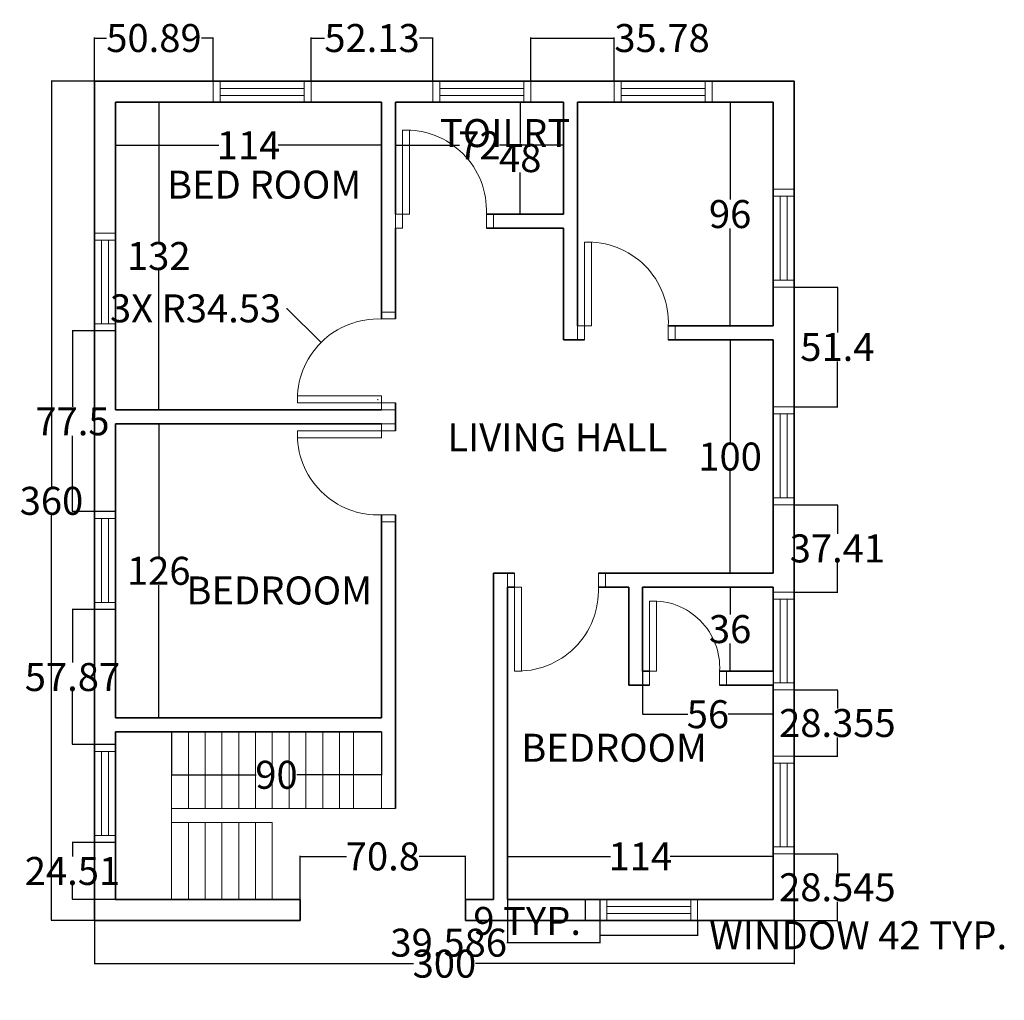
# Model space of a CAD drawing. Units: inches. Extents: x -24 to 1692, y -109 to 592.
# Tile 4 of 4: x 1270 to 1692, y 17 to 437. Entities that reach past the tile are written whole.
import ezdxf
from ezdxf.enums import TextEntityAlignment as Align

# ---------------------------------------------------------------- set-up
doc = ezdxf.new("R2010")
doc.units = ezdxf.units.IN
doc.header["$MEASUREMENT"] = 0
for name, color, linetype, lineweight in [('A-ANNO-DIMS', 2, 'Continuous', 18), ('A-AREA-IDEN', 7, 'Continuous', 18), ('A-DOOR', 3, 'Continuous', 18), ('A-FLOR-STRS', 2, 'Continuous', 18), ('A-GLAZ', 4, 'Continuous', 18), ('A-WALL', 7, 'Continuous', 35)]:
    doc.layers.add(name, color=color, linetype=linetype, lineweight=lineweight)
doc.styles.get("Standard").update_dxf_attribs({"font": 'arial.ttf'})
doc.dimstyles.get("Standard").update_dxf_attribs({"dimtxt": 12, "dimasz": 0.18, "dimexe": 0.18, "dimexo": 0.0625, "dimgap": 0.09, "dimtad": 0, "dimtih": 1, "dimtoh": 1, "dimdec": 0, "dimzin": 0, "dimdsep": 46, "dimlunit": 4, "dimtxsty": 'Standard', "dimcen": 0.09, "dimadec": 0, "dimazin": 0, "dimtfac": 1, "dimtdec": 0, "dimtofl": 0, "dimtmove": 0, "dimatfit": 3, "dimfxl": 1, "dimtolj": 1, "dimtzin": 0, "dimarcsym": 0})

# ---------------------------------------------------------------- blocks, each defined once
blk = doc.blocks.new('K')
for p, q in [((0, 42), (9, 42)), ((0, 3), (0, 39)), ((0, 39), (9, 39)), ((3, 3), (3, 39)), ((6, 39), (6, 3)), ((9, 39), (9, 3)), ((9, 3), (0, 3)), ((9, 0), (0, 0))]:
    blk.add_line(p, q)
blk = doc.blocks.new('DOOR-SWING-36IN')
for p, q in [((-39, 0), (-39, 6)), ((-36, 0), (-36, 6)), ((0, 0), (0, 6)), ((3, 0), (3, 6))]:
    blk.add_line(p, q)
blk.add_lwpolyline([(0, 0), (-3, 0), (-3, -36), (0, -36)], close=True)
blk.add_arc((-1.5, -1.5), 34.53, 177.5104, 272.4896)
blk = doc.blocks.new('DOOR-SWING-30IN')
for p, q in [((-3, 6), (-3, 0)), ((0, 6), (0, 0)), ((30, 6), (30, 0)), ((33, 6), (33, 0))]:
    blk.add_line(p, q)
blk.add_lwpolyline([(0, 0), (3, 0), (3, -30), (0, -30)], close=True)
blk.add_arc((1.5, -1.5), 28.54, 266.9872, 3.0128)
blk = doc.blocks.new('*D5')
at = {"layer": 'A-ANNO-DIMS', "color": 0, "lineweight": -2, "transparency": 16777216}
for p, q in [((1519, 51.05), (1519, 44.64)), ((1561, 51.05), (1561, 44.64)), ((1519.18, 44.82), (1560.82, 44.82)), ((1561, 44.82), (1561.18, 44.82))]:
    blk.add_line(p, q, dxfattribs=at)
at = {"layer": 'A-ANNO-DIMS', "color": 0, "transparency": 16777216}
for points in [[(1519.18, 44.85), (1519.18, 44.79), (1519, 44.82)], [(1560.82, 44.85), (1560.82, 44.79), (1561, 44.82)]]:
    blk.add_solid(points, dxfattribs=at)
at = {"layer": 'Defpoints', "color": 0, "transparency": 16777216}
for p in [(1519, 51.12), (1561, 51.12), (1561, 44.82)]:
    blk.add_point(p, dxfattribs=at)
at = {"layer": 'A-ANNO-DIMS', "color": 0, "transparency": 16777216, "insert": (1629.83, 44.82), "char_height": 12, "attachment_point": 5}
blk.add_mtext('\\A1;WINDOW 42 TYP.', dxfattribs=at)
blk = doc.blocks.new('*D6')
at = {"layer": 'A-ANNO-DIMS', "color": 0, "lineweight": -2, "transparency": 16777216}
for p, q in [((1518.94, 60.12), (1512.52, 60.12)), ((1512.7, 59.94), (1512.7, 51.3)), ((1518.94, 51.12), (1512.52, 51.12)), ((1512.7, 50.94), (1512.52, 50.94)), ((1512.7, 51.12), (1512.7, 50.94))]:
    blk.add_line(p, q, dxfattribs=at)
at = {"layer": 'A-ANNO-DIMS', "color": 0, "transparency": 16777216}
for points in [[(1512.67, 59.94), (1512.73, 59.94), (1512.7, 60.12)], [(1512.67, 51.3), (1512.73, 51.3), (1512.7, 51.12)]]:
    blk.add_solid(points, dxfattribs=at)
at = {"layer": 'Defpoints', "color": 0, "transparency": 16777216}
for p in [(1519, 60.12), (1512.7, 51.12), (1519, 51.12)]:
    blk.add_point(p, dxfattribs=at)
at = {"layer": 'A-ANNO-DIMS', "color": 0, "transparency": 16777216, "insert": (1487.89, 50.94), "char_height": 12, "attachment_point": 5}
blk.add_mtext('\\A1;9 TYP.', dxfattribs=at)
blk = doc.blocks.new('*D72')
at = {"layer": 'A-ANNO-DIMS', "color": 0, "lineweight": -2, "transparency": 16777216}
for p, q in [((1302.41, 51.05), (1302.41, 32.44)), ((1602.41, 51.05), (1602.41, 32.44)), ((1302.59, 32.62), (1439.09, 32.62)), ((1602.23, 32.62), (1465.74, 32.62))]:
    blk.add_line(p, q, dxfattribs=at)
at = {"layer": 'A-ANNO-DIMS', "color": 0, "transparency": 16777216}
for points in [[(1302.59, 32.65), (1302.59, 32.59), (1302.41, 32.62)], [(1602.23, 32.65), (1602.23, 32.59), (1602.41, 32.62)]]:
    blk.add_solid(points, dxfattribs=at)
at = {"layer": 'Defpoints', "color": 0, "transparency": 16777216}
for p in [(1302.41, 51.12), (1602.41, 51.12), (1602.41, 32.62)]:
    blk.add_point(p, dxfattribs=at)
at = {"layer": 'A-ANNO-DIMS', "color": 0, "transparency": 16777216, "insert": (1452.41, 32.62), "char_height": 12, "attachment_point": 5}
blk.add_mtext('\\A1;300', dxfattribs=at)
blk = doc.blocks.new('*D73')
at = {"layer": 'A-ANNO-DIMS', "color": 0, "lineweight": -2, "transparency": 16777216}
for p, q in [((1302.35, 411.12), (1283.73, 411.12)), ((1283.91, 410.94), (1283.91, 237.34)), ((1283.91, 51.3), (1283.91, 224.89)), ((1302.35, 51.12), (1283.73, 51.12))]:
    blk.add_line(p, q, dxfattribs=at)
at = {"layer": 'A-ANNO-DIMS', "color": 0, "transparency": 16777216}
for points in [[(1283.88, 410.94), (1283.94, 410.94), (1283.91, 411.12)], [(1283.88, 51.3), (1283.94, 51.3), (1283.91, 51.12)]]:
    blk.add_solid(points, dxfattribs=at)
at = {"layer": 'Defpoints', "color": 0, "transparency": 16777216}
for p in [(1283.91, 411.12), (1302.41, 411.12), (1302.41, 51.12)]:
    blk.add_point(p, dxfattribs=at)
at = {"layer": 'A-ANNO-DIMS', "color": 0, "transparency": 16777216, "insert": (1283.91, 231.12), "char_height": 12, "attachment_point": 5}
blk.add_mtext('\\A1;360', dxfattribs=at)
blk = doc.blocks.new('*D74')
at = {"layer": 'A-ANNO-DIMS', "color": 0, "lineweight": -2, "transparency": 16777216}
for p, q in [((1311.41, 402.05), (1311.41, 383.44)), ((1425.41, 402.05), (1425.41, 383.44)), ((1311.59, 383.62), (1355.66, 383.62)), ((1425.23, 383.62), (1381.17, 383.62))]:
    blk.add_line(p, q, dxfattribs=at)
at = {"layer": 'A-ANNO-DIMS', "color": 0, "transparency": 16777216}
for points in [[(1311.59, 383.65), (1311.59, 383.59), (1311.41, 383.62)], [(1425.23, 383.65), (1425.23, 383.59), (1425.41, 383.62)]]:
    blk.add_solid(points, dxfattribs=at)
at = {"layer": 'Defpoints', "color": 0, "transparency": 16777216}
for p in [(1311.41, 402.12), (1425.41, 402.12), (1311.41, 383.62)]:
    blk.add_point(p, dxfattribs=at)
at = {"layer": 'A-ANNO-DIMS', "color": 0, "transparency": 16777216, "insert": (1368.41, 383.62), "char_height": 12, "attachment_point": 5}
blk.add_mtext('\\A1;114', dxfattribs=at)
blk = doc.blocks.new('*D75')
at = {"layer": 'A-ANNO-DIMS', "color": 0, "lineweight": -2, "transparency": 16777216}
for p, q in [((1431.41, 402.05), (1431.41, 383.44)), ((1503.41, 402.05), (1503.41, 383.44)), ((1431.59, 383.62), (1458.84, 383.62)), ((1503.23, 383.62), (1475.99, 383.62))]:
    blk.add_line(p, q, dxfattribs=at)
at = {"layer": 'A-ANNO-DIMS', "color": 0, "transparency": 16777216}
for points in [[(1431.59, 383.65), (1431.59, 383.59), (1431.41, 383.62)], [(1503.23, 383.65), (1503.23, 383.59), (1503.41, 383.62)]]:
    blk.add_solid(points, dxfattribs=at)
at = {"layer": 'Defpoints', "color": 0, "transparency": 16777216}
for p in [(1431.41, 402.12), (1503.41, 402.12), (1431.41, 383.62)]:
    blk.add_point(p, dxfattribs=at)
at = {"layer": 'A-ANNO-DIMS', "color": 0, "transparency": 16777216, "insert": (1467.41, 383.62), "char_height": 12, "attachment_point": 5}
blk.add_mtext('\\A1;72', dxfattribs=at)
blk = doc.blocks.new('*D76')
at = {"layer": 'A-ANNO-DIMS', "color": 0, "lineweight": -2, "transparency": 16777216}
for p, q in [((1311.48, 402.12), (1330.09, 402.12)), ((1329.91, 401.94), (1329.91, 342.34)), ((1329.91, 270.3), (1329.91, 329.89)), ((1311.48, 270.12), (1330.09, 270.12))]:
    blk.add_line(p, q, dxfattribs=at)
at = {"layer": 'A-ANNO-DIMS', "color": 0, "transparency": 16777216}
for points in [[(1329.88, 401.94), (1329.94, 401.94), (1329.91, 402.12)], [(1329.88, 270.3), (1329.94, 270.3), (1329.91, 270.12)]]:
    blk.add_solid(points, dxfattribs=at)
at = {"layer": 'Defpoints', "color": 0, "transparency": 16777216}
for p in [(1311.41, 402.12), (1311.41, 270.12), (1329.91, 270.12)]:
    blk.add_point(p, dxfattribs=at)
at = {"layer": 'A-ANNO-DIMS', "color": 0, "transparency": 16777216, "insert": (1329.91, 336.12), "char_height": 12, "attachment_point": 5}
blk.add_mtext('\\A1;132', dxfattribs=at)
blk = doc.blocks.new('*D77')
at = {"layer": 'A-ANNO-DIMS', "color": 0, "lineweight": -2, "transparency": 16777216}
for p, q in [((1311.48, 264.12), (1330.09, 264.12)), ((1329.91, 263.94), (1329.91, 207.33)), ((1329.91, 138.3), (1329.91, 194.9)), ((1311.48, 138.12), (1330.09, 138.12))]:
    blk.add_line(p, q, dxfattribs=at)
at = {"layer": 'A-ANNO-DIMS', "color": 0, "transparency": 16777216}
for points in [[(1329.88, 263.94), (1329.94, 263.94), (1329.91, 264.12)], [(1329.88, 138.3), (1329.94, 138.3), (1329.91, 138.12)]]:
    blk.add_solid(points, dxfattribs=at)
at = {"layer": 'Defpoints', "color": 0, "transparency": 16777216}
for p in [(1311.41, 264.12), (1311.41, 138.12), (1329.91, 138.12)]:
    blk.add_point(p, dxfattribs=at)
at = {"layer": 'A-ANNO-DIMS', "color": 0, "transparency": 16777216, "insert": (1329.91, 201.12), "char_height": 12, "attachment_point": 5}
blk.add_mtext('\\A1;126', dxfattribs=at)
blk = doc.blocks.new('*D78')
at = {"layer": 'A-ANNO-DIMS', "color": 0, "lineweight": -2, "transparency": 16777216}
for p, q in [((1593.35, 402.12), (1574.73, 402.12)), ((1574.91, 401.94), (1574.91, 360.33)), ((1574.91, 306.3), (1574.91, 347.9)), ((1593.35, 306.12), (1574.73, 306.12))]:
    blk.add_line(p, q, dxfattribs=at)
at = {"layer": 'A-ANNO-DIMS', "color": 0, "transparency": 16777216}
for points in [[(1574.88, 401.94), (1574.94, 401.94), (1574.91, 402.12)], [(1574.88, 306.3), (1574.94, 306.3), (1574.91, 306.12)]]:
    blk.add_solid(points, dxfattribs=at)
at = {"layer": 'Defpoints', "color": 0, "transparency": 16777216}
for p in [(1574.91, 402.12), (1593.41, 402.12), (1593.41, 306.12)]:
    blk.add_point(p, dxfattribs=at)
at = {"layer": 'A-ANNO-DIMS', "color": 0, "transparency": 16777216, "insert": (1574.91, 354.12), "char_height": 12, "attachment_point": 5}
blk.add_mtext('\\A1;96', dxfattribs=at)
blk = doc.blocks.new('*D79')
at = {"layer": 'A-ANNO-DIMS', "color": 0, "lineweight": -2, "transparency": 16777216}
for p, q in [((1593.35, 300.12), (1574.73, 300.12)), ((1574.91, 299.94), (1574.91, 256.33)), ((1574.91, 200.3), (1574.91, 243.9)), ((1593.35, 200.12), (1574.73, 200.12))]:
    blk.add_line(p, q, dxfattribs=at)
at = {"layer": 'A-ANNO-DIMS', "color": 0, "transparency": 16777216}
for points in [[(1574.88, 299.94), (1574.94, 299.94), (1574.91, 300.12)], [(1574.88, 200.3), (1574.94, 200.3), (1574.91, 200.12)]]:
    blk.add_solid(points, dxfattribs=at)
at = {"layer": 'Defpoints', "color": 0, "transparency": 16777216}
for p in [(1574.91, 300.12), (1593.41, 300.12), (1593.41, 200.12)]:
    blk.add_point(p, dxfattribs=at)
at = {"layer": 'A-ANNO-DIMS', "color": 0, "transparency": 16777216, "insert": (1574.91, 250.12), "char_height": 12, "attachment_point": 5}
blk.add_mtext('\\A1;100', dxfattribs=at)
blk = doc.blocks.new('*D80')
at = {"layer": 'A-ANNO-DIMS', "color": 0, "lineweight": -2, "transparency": 16777216}
for p, q in [((1503.35, 402.12), (1484.73, 402.12)), ((1484.91, 401.94), (1484.91, 384.33)), ((1484.91, 354.3), (1484.91, 371.9)), ((1503.35, 354.12), (1484.73, 354.12))]:
    blk.add_line(p, q, dxfattribs=at)
at = {"layer": 'A-ANNO-DIMS', "color": 0, "transparency": 16777216}
for points in [[(1484.88, 401.94), (1484.94, 401.94), (1484.91, 402.12)], [(1484.88, 354.3), (1484.94, 354.3), (1484.91, 354.12)]]:
    blk.add_solid(points, dxfattribs=at)
at = {"layer": 'Defpoints', "color": 0, "transparency": 16777216}
for p in [(1484.91, 402.12), (1503.41, 402.12), (1503.41, 354.12)]:
    blk.add_point(p, dxfattribs=at)
at = {"layer": 'A-ANNO-DIMS', "color": 0, "transparency": 16777216, "insert": (1484.91, 378.12), "char_height": 12, "attachment_point": 5}
blk.add_mtext('\\A1;48', dxfattribs=at)
blk = doc.blocks.new('*D81')
at = {"layer": 'A-ANNO-DIMS', "color": 0, "lineweight": -2, "transparency": 16777216}
for p, q in [((1479.41, 60.18), (1479.41, 78.8)), ((1479.59, 78.62), (1523.66, 78.62)), ((1593.23, 78.62), (1549.17, 78.62)), ((1593.41, 60.18), (1593.41, 78.8))]:
    blk.add_line(p, q, dxfattribs=at)
at = {"layer": 'A-ANNO-DIMS', "color": 0, "transparency": 16777216}
for points in [[(1479.59, 78.65), (1479.59, 78.59), (1479.41, 78.62)], [(1593.23, 78.65), (1593.23, 78.59), (1593.41, 78.62)]]:
    blk.add_solid(points, dxfattribs=at)
at = {"layer": 'Defpoints', "color": 0, "transparency": 16777216}
for p in [(1593.41, 78.62), (1479.41, 60.12), (1593.41, 60.12)]:
    blk.add_point(p, dxfattribs=at)
at = {"layer": 'A-ANNO-DIMS', "color": 0, "transparency": 16777216, "insert": (1536.41, 78.62), "char_height": 12, "attachment_point": 5}
blk.add_mtext('\\A1;114', dxfattribs=at)
blk = doc.blocks.new('*D82')
at = {"layer": 'A-ANNO-DIMS', "color": 0, "lineweight": -2, "transparency": 16777216}
for p, q in [((1390.61, 60.18), (1390.61, 78.8)), ((1390.79, 78.62), (1410.38, 78.62)), ((1461.23, 78.62), (1441.65, 78.62)), ((1461.41, 60.18), (1461.41, 78.8))]:
    blk.add_line(p, q, dxfattribs=at)
at = {"layer": 'A-ANNO-DIMS', "color": 0, "transparency": 16777216}
for points in [[(1390.79, 78.65), (1390.79, 78.59), (1390.61, 78.62)], [(1461.23, 78.65), (1461.23, 78.59), (1461.41, 78.62)]]:
    blk.add_solid(points, dxfattribs=at)
at = {"layer": 'Defpoints', "color": 0, "transparency": 16777216}
for p in [(1461.41, 78.62), (1390.61, 60.12), (1461.41, 60.12)]:
    blk.add_point(p, dxfattribs=at)
at = {"layer": 'A-ANNO-DIMS', "color": 0, "transparency": 16777216, "insert": (1426.01, 78.62), "char_height": 12, "attachment_point": 5}
blk.add_mtext('\\A1;70.8', dxfattribs=at)
blk = doc.blocks.new('*D83')
at = {"layer": 'A-ANNO-DIMS', "color": 0, "lineweight": -2, "transparency": 16777216}
for p, q in [((1537.41, 158.05), (1537.41, 139.44)), ((1593.41, 158.05), (1593.41, 139.44)), ((1537.59, 139.62), (1556.73, 139.62)), ((1593.23, 139.62), (1574.09, 139.62))]:
    blk.add_line(p, q, dxfattribs=at)
at = {"layer": 'A-ANNO-DIMS', "color": 0, "transparency": 16777216}
for points in [[(1537.59, 139.65), (1537.59, 139.59), (1537.41, 139.62)], [(1593.23, 139.65), (1593.23, 139.59), (1593.41, 139.62)]]:
    blk.add_solid(points, dxfattribs=at)
at = {"layer": 'Defpoints', "color": 0, "transparency": 16777216}
for p in [(1537.41, 158.12), (1593.41, 158.12), (1537.41, 139.62)]:
    blk.add_point(p, dxfattribs=at)
at = {"layer": 'A-ANNO-DIMS', "color": 0, "transparency": 16777216, "insert": (1565.41, 139.62), "char_height": 12, "attachment_point": 5}
blk.add_mtext('\\A1;56', dxfattribs=at)
blk = doc.blocks.new('*D84')
at = {"layer": 'A-ANNO-DIMS', "color": 0, "lineweight": -2, "transparency": 16777216}
for p, q in [((1593.35, 194.12), (1574.73, 194.12)), ((1574.91, 193.94), (1574.91, 182.34)), ((1574.91, 158.3), (1574.91, 169.89)), ((1593.35, 158.12), (1574.73, 158.12))]:
    blk.add_line(p, q, dxfattribs=at)
at = {"layer": 'A-ANNO-DIMS', "color": 0, "transparency": 16777216}
for points in [[(1574.88, 193.94), (1574.94, 193.94), (1574.91, 194.12)], [(1574.88, 158.3), (1574.94, 158.3), (1574.91, 158.12)]]:
    blk.add_solid(points, dxfattribs=at)
at = {"layer": 'Defpoints', "color": 0, "transparency": 16777216}
for p in [(1574.91, 194.12), (1593.41, 194.12), (1593.41, 158.12)]:
    blk.add_point(p, dxfattribs=at)
at = {"layer": 'A-ANNO-DIMS', "color": 0, "transparency": 16777216, "insert": (1574.91, 176.12), "char_height": 12, "attachment_point": 5}
blk.add_mtext('\\A1;36', dxfattribs=at)
blk = doc.blocks.new('*D85')
at = {"layer": 'A-ANNO-DIMS', "color": 0, "lineweight": -2, "transparency": 16777216}
for p, q in [((1302.41, 411.18), (1302.41, 429.8)), ((1302.59, 429.62), (1307.51, 429.62)), ((1353.12, 429.62), (1348.21, 429.62)), ((1353.3, 411.07), (1353.3, 429.8))]:
    blk.add_line(p, q, dxfattribs=at)
at = {"layer": 'A-ANNO-DIMS', "color": 0, "transparency": 16777216}
for points in [[(1302.59, 429.65), (1302.59, 429.59), (1302.41, 429.62)], [(1353.12, 429.65), (1353.12, 429.59), (1353.3, 429.62)]]:
    blk.add_solid(points, dxfattribs=at)
at = {"layer": 'Defpoints', "color": 0, "transparency": 16777216}
for p in [(1353.3, 429.62), (1302.41, 411.12), (1353.3, 411.01)]:
    blk.add_point(p, dxfattribs=at)
at = {"layer": 'A-ANNO-DIMS', "color": 0, "transparency": 16777216, "insert": (1327.86, 429.62), "char_height": 12, "attachment_point": 5}
blk.add_mtext('\\A1;50.89', dxfattribs=at)
blk = doc.blocks.new('*D86')
at = {"layer": 'A-ANNO-DIMS', "color": 0, "lineweight": -2, "transparency": 16777216}
for p, q in [((1395.3, 411.07), (1395.3, 429.8)), ((1395.48, 429.62), (1401.03, 429.62)), ((1447.25, 429.62), (1441.71, 429.62)), ((1447.43, 411.07), (1447.43, 429.8))]:
    blk.add_line(p, q, dxfattribs=at)
at = {"layer": 'A-ANNO-DIMS', "color": 0, "transparency": 16777216}
for points in [[(1395.48, 429.65), (1395.48, 429.59), (1395.3, 429.62)], [(1447.25, 429.65), (1447.25, 429.59), (1447.43, 429.62)]]:
    blk.add_solid(points, dxfattribs=at)
at = {"layer": 'Defpoints', "color": 0, "transparency": 16777216}
for p in [(1447.43, 429.62), (1395.3, 411.01), (1447.43, 411.01)]:
    blk.add_point(p, dxfattribs=at)
at = {"layer": 'A-ANNO-DIMS', "color": 0, "transparency": 16777216, "insert": (1421.37, 429.62), "char_height": 12, "attachment_point": 5}
blk.add_mtext('\\A1;52.13', dxfattribs=at)
blk = doc.blocks.new('*D87')
at = {"layer": 'A-ANNO-DIMS', "color": 0, "lineweight": -2, "transparency": 16777216}
for p, q in [((1489.43, 411.07), (1489.43, 429.8)), ((1489.61, 429.62), (1525.04, 429.62)), ((1525.22, 411.07), (1525.22, 429.8)), ((1525.22, 429.62), (1525.4, 429.62))]:
    blk.add_line(p, q, dxfattribs=at)
at = {"layer": 'A-ANNO-DIMS', "color": 0, "transparency": 16777216}
for points in [[(1489.61, 429.65), (1489.61, 429.59), (1489.43, 429.62)], [(1525.04, 429.65), (1525.04, 429.59), (1525.22, 429.62)]]:
    blk.add_solid(points, dxfattribs=at)
at = {"layer": 'Defpoints', "color": 0, "transparency": 16777216}
for p in [(1525.22, 429.62), (1489.43, 411.01), (1525.22, 411.01)]:
    blk.add_point(p, dxfattribs=at)
at = {"layer": 'A-ANNO-DIMS', "color": 0, "transparency": 16777216, "insert": (1545.74, 429.62), "char_height": 12, "attachment_point": 5}
blk.add_mtext('\\A1;35.78', dxfattribs=at)
blk = doc.blocks.new('*D88')
at = {"layer": 'A-ANNO-DIMS', "color": 0, "lineweight": -2, "transparency": 16777216}
for p, q in [((1311.35, 84.62), (1292.73, 84.62)), ((1292.91, 84.44), (1292.91, 78.59)), ((1292.91, 60.3), (1292.91, 66.15)), ((1311.35, 60.12), (1292.73, 60.12))]:
    blk.add_line(p, q, dxfattribs=at)
at = {"layer": 'A-ANNO-DIMS', "color": 0, "transparency": 16777216}
for points in [[(1292.88, 84.44), (1292.94, 84.44), (1292.91, 84.62)], [(1292.88, 60.3), (1292.94, 60.3), (1292.91, 60.12)]]:
    blk.add_solid(points, dxfattribs=at)
at = {"layer": 'Defpoints', "color": 0, "transparency": 16777216}
for p in [(1292.91, 84.62), (1311.41, 84.62), (1311.41, 60.12)]:
    blk.add_point(p, dxfattribs=at)
at = {"layer": 'A-ANNO-DIMS', "color": 0, "transparency": 16777216, "insert": (1292.91, 72.37), "char_height": 12, "attachment_point": 5}
blk.add_mtext('\\A1;24.51', dxfattribs=at)
blk = doc.blocks.new('*D89')
at = {"layer": 'A-ANNO-DIMS', "color": 0, "lineweight": -2, "transparency": 16777216}
for p, q in [((1311.35, 184.5), (1292.73, 184.5)), ((1292.91, 184.32), (1292.91, 161.78)), ((1292.91, 126.8), (1292.91, 149.34)), ((1311.35, 126.62), (1292.73, 126.62))]:
    blk.add_line(p, q, dxfattribs=at)
at = {"layer": 'A-ANNO-DIMS', "color": 0, "transparency": 16777216}
for points in [[(1292.88, 184.32), (1292.94, 184.32), (1292.91, 184.5)], [(1292.88, 126.8), (1292.94, 126.8), (1292.91, 126.62)]]:
    blk.add_solid(points, dxfattribs=at)
at = {"layer": 'Defpoints', "color": 0, "transparency": 16777216}
for p in [(1292.91, 184.5), (1311.41, 184.5), (1311.41, 126.62)]:
    blk.add_point(p, dxfattribs=at)
at = {"layer": 'A-ANNO-DIMS', "color": 0, "transparency": 16777216, "insert": (1292.91, 155.56), "char_height": 12, "attachment_point": 5}
blk.add_mtext('\\A1;57.87', dxfattribs=at)
blk = doc.blocks.new('*D90')
at = {"layer": 'A-ANNO-DIMS', "color": 0, "lineweight": -2, "transparency": 16777216}
for p, q in [((1311.35, 303.99), (1292.73, 303.99)), ((1292.91, 303.81), (1292.91, 271.44)), ((1292.91, 226.68), (1292.91, 259.05)), ((1311.35, 226.5), (1292.73, 226.5))]:
    blk.add_line(p, q, dxfattribs=at)
at = {"layer": 'A-ANNO-DIMS', "color": 0, "transparency": 16777216}
for points in [[(1292.88, 303.81), (1292.94, 303.81), (1292.91, 303.99)], [(1292.88, 226.68), (1292.94, 226.68), (1292.91, 226.5)]]:
    blk.add_solid(points, dxfattribs=at)
at = {"layer": 'Defpoints', "color": 0, "transparency": 16777216}
for p in [(1292.91, 303.99), (1311.41, 303.99), (1311.41, 226.5)]:
    blk.add_point(p, dxfattribs=at)
at = {"layer": 'A-ANNO-DIMS', "color": 0, "transparency": 16777216, "insert": (1292.91, 265.24), "char_height": 12, "attachment_point": 5}
blk.add_mtext('\\A1;77.5', dxfattribs=at)
blk = doc.blocks.new('*D91')
at = {"layer": 'A-ANNO-DIMS', "color": 0, "lineweight": -2, "transparency": 16777216}
for p, q in [((1602.48, 79.66), (1621.09, 79.66)), ((1620.91, 79.48), (1620.91, 71.6)), ((1620.91, 51.3), (1620.91, 59.17)), ((1602.48, 51.12), (1621.09, 51.12))]:
    blk.add_line(p, q, dxfattribs=at)
at = {"layer": 'A-ANNO-DIMS', "color": 0, "transparency": 16777216}
for points in [[(1620.88, 79.48), (1620.94, 79.48), (1620.91, 79.66)], [(1620.88, 51.3), (1620.94, 51.3), (1620.91, 51.12)]]:
    blk.add_solid(points, dxfattribs=at)
at = {"layer": 'Defpoints', "color": 0, "transparency": 16777216}
for p in [(1602.41, 79.66), (1620.91, 79.66), (1602.41, 51.12)]:
    blk.add_point(p, dxfattribs=at)
at = {"layer": 'A-ANNO-DIMS', "color": 0, "transparency": 16777216, "insert": (1620.91, 65.39), "char_height": 12, "attachment_point": 5}
blk.add_mtext('\\A1;28.545', dxfattribs=at)
blk = doc.blocks.new('*D92')
at = {"layer": 'A-ANNO-DIMS', "color": 0, "lineweight": -2, "transparency": 16777216}
for p, q in [((1602.48, 150.02), (1621.09, 150.02)), ((1620.91, 149.84), (1620.91, 142.06)), ((1620.91, 121.84), (1620.91, 129.62)), ((1602.48, 121.66), (1621.09, 121.66))]:
    blk.add_line(p, q, dxfattribs=at)
at = {"layer": 'A-ANNO-DIMS', "color": 0, "transparency": 16777216}
for points in [[(1620.88, 149.84), (1620.94, 149.84), (1620.91, 150.02)], [(1620.88, 121.84), (1620.94, 121.84), (1620.91, 121.66)]]:
    blk.add_solid(points, dxfattribs=at)
at = {"layer": 'Defpoints', "color": 0, "transparency": 16777216}
for p in [(1602.41, 150.02), (1620.91, 150.02), (1602.41, 121.66)]:
    blk.add_point(p, dxfattribs=at)
at = {"layer": 'A-ANNO-DIMS', "color": 0, "transparency": 16777216, "insert": (1620.91, 135.84), "char_height": 12, "attachment_point": 5}
blk.add_mtext('\\A1;28.355', dxfattribs=at)
blk = doc.blocks.new('*D93')
at = {"layer": 'A-ANNO-DIMS', "color": 0, "lineweight": -2, "transparency": 16777216}
for p, q in [((1602.48, 229.42), (1621.09, 229.42)), ((1620.91, 229.24), (1620.91, 216.94)), ((1620.91, 192.2), (1620.91, 204.5)), ((1602.48, 192.02), (1621.09, 192.02))]:
    blk.add_line(p, q, dxfattribs=at)
at = {"layer": 'A-ANNO-DIMS', "color": 0, "transparency": 16777216}
for points in [[(1620.88, 229.24), (1620.94, 229.24), (1620.91, 229.42)], [(1620.88, 192.2), (1620.94, 192.2), (1620.91, 192.02)]]:
    blk.add_solid(points, dxfattribs=at)
at = {"layer": 'Defpoints', "color": 0, "transparency": 16777216}
for p in [(1602.41, 229.42), (1620.91, 229.42), (1602.41, 192.02)]:
    blk.add_point(p, dxfattribs=at)
at = {"layer": 'A-ANNO-DIMS', "color": 0, "transparency": 16777216, "insert": (1620.91, 210.72), "char_height": 12, "attachment_point": 5}
blk.add_mtext('\\A1;37.41', dxfattribs=at)
blk = doc.blocks.new('*D94')
at = {"layer": 'A-ANNO-DIMS', "color": 0, "lineweight": -2, "transparency": 16777216}
for p, q in [((1602.48, 322.83), (1621.09, 322.83)), ((1620.91, 322.65), (1620.91, 303.34)), ((1620.91, 271.6), (1620.91, 290.91)), ((1602.48, 271.42), (1621.09, 271.42))]:
    blk.add_line(p, q, dxfattribs=at)
at = {"layer": 'A-ANNO-DIMS', "color": 0, "transparency": 16777216}
for points in [[(1620.88, 322.65), (1620.94, 322.65), (1620.91, 322.83)], [(1620.88, 271.6), (1620.94, 271.6), (1620.91, 271.42)]]:
    blk.add_solid(points, dxfattribs=at)
at = {"layer": 'Defpoints', "color": 0, "transparency": 16777216}
for p in [(1602.41, 322.83), (1620.91, 322.83), (1602.41, 271.42)]:
    blk.add_point(p, dxfattribs=at)
at = {"layer": 'A-ANNO-DIMS', "color": 0, "transparency": 16777216, "insert": (1620.91, 297.13), "char_height": 12, "attachment_point": 5}
blk.add_mtext('\\A1;51.4', dxfattribs=at)
blk = doc.blocks.new('*D95')
at = {"layer": 'A-ANNO-DIMS', "color": 0, "lineweight": -2, "transparency": 16777216}
for p, q in [((1479.41, 60.05), (1479.41, 41.44)), ((1519, 60.05), (1519, 41.44)), ((1479.41, 41.62), (1479.23, 41.62)), ((1518.82, 41.62), (1479.59, 41.62))]:
    blk.add_line(p, q, dxfattribs=at)
at = {"layer": 'A-ANNO-DIMS', "color": 0, "transparency": 16777216}
for points in [[(1479.59, 41.65), (1479.59, 41.59), (1479.41, 41.62)], [(1518.82, 41.65), (1518.82, 41.59), (1519, 41.62)]]:
    blk.add_solid(points, dxfattribs=at)
at = {"layer": 'Defpoints', "color": 0, "transparency": 16777216}
for p in [(1479.41, 60.12), (1519, 60.12), (1479.41, 41.62)]:
    blk.add_point(p, dxfattribs=at)
at = {"layer": 'A-ANNO-DIMS', "color": 0, "transparency": 16777216, "insert": (1454.24, 41.62), "char_height": 12, "attachment_point": 5}
blk.add_mtext('\\A1;39.586', dxfattribs=at)
blk = doc.blocks.new('*D96')
at = {"layer": 'A-ANNO-DIMS', "color": 0, "lineweight": -2, "transparency": 16777216}
for p, q in [((1335.41, 132.05), (1335.41, 113.44)), ((1425.41, 132.05), (1425.41, 113.44)), ((1335.59, 113.62), (1371.75, 113.62)), ((1425.23, 113.62), (1389.08, 113.62))]:
    blk.add_line(p, q, dxfattribs=at)
at = {"layer": 'A-ANNO-DIMS', "color": 0, "transparency": 16777216}
for points in [[(1335.59, 113.65), (1335.59, 113.59), (1335.41, 113.62)], [(1425.23, 113.65), (1425.23, 113.59), (1425.41, 113.62)]]:
    blk.add_solid(points, dxfattribs=at)
at = {"layer": 'Defpoints', "color": 0, "transparency": 16777216}
for p in [(1335.41, 132.12), (1425.41, 132.12), (1335.41, 113.62)]:
    blk.add_point(p, dxfattribs=at)
at = {"layer": 'A-ANNO-DIMS', "color": 0, "transparency": 16777216, "insert": (1380.41, 113.62), "char_height": 12, "attachment_point": 5}
blk.add_mtext('\\A1;90', dxfattribs=at)
blk = doc.blocks.new('*D100')
at = {"layer": 'A-ANNO-DIMS', "color": 0, "lineweight": -2, "transparency": 16777216}
for p, q in [((1384.66, 313.68), (1384.84, 313.68)), ((1384.84, 313.68), (1399.37, 299.16)), ((1423.82, 274.62), (1424, 274.62)), ((1423.91, 274.53), (1423.91, 274.71))]:
    blk.add_line(p, q, dxfattribs=at)
at = {"layer": 'A-ANNO-DIMS', "color": 0, "transparency": 16777216}
blk.add_solid([(1399.39, 299.18), (1399.35, 299.14), (1399.5, 299.03)], dxfattribs=at)
at = {"layer": 'Defpoints', "color": 0, "transparency": 16777216}
for p in [(1399.5, 299.03), (1423.91, 274.62)]:
    blk.add_point(p, dxfattribs=at)
at = {"layer": 'A-ANNO-DIMS', "color": 0, "transparency": 16777216, "insert": (1345.7, 313.68), "char_height": 12, "attachment_point": 5}
blk.add_mtext('\\A1;3X R34.53', dxfattribs=at)

msp = doc.modelspace()

# ---------------------------------------------------------------- linework, layer by layer
at = {"layer": 'A-DOOR'}
for p, q in [((1434.4142, 354.1152), (1431.4142, 354.1152)), ((1434.4142, 348.1152), (1431.4142, 348.1152)), ((1512.4142, 306.1152), (1509.4142, 306.1152)), ((1425.4142, 270.1152), (1425.4142, 273.1152)), ((1425.4142, 261.1152), (1425.4142, 264.1152))]:
    msp.add_line(p, q, dxfattribs=at)
at = {"layer": 'A-FLOR-STRS'}
for p, q in [((1335.4142, 132.1152), (1335.4142, 60.1152)), ((1342.6142, 132.1152), (1342.6142, 99.1152)), ((1349.8142, 132.1152), (1349.8142, 99.1152)), ((1357.0142, 132.1152), (1357.0142, 99.1152)), ((1364.2142, 132.1152), (1364.2142, 99.1152)), ((1371.4142, 132.1152), (1371.4142, 99.1152)), ((1378.6142, 132.1152), (1378.6142, 99.1152)), ((1385.8142, 132.1152), (1385.8142, 99.1152)), ((1393.0142, 132.1152), (1393.0142, 99.1152)), ((1400.2142, 132.1152), (1400.2142, 99.1152)), ((1407.4142, 132.1152), (1407.4142, 99.1152)), ((1413.4142, 99.1152), (1413.4142, 132.1152)), ((1425.4142, 99.1152), (1425.4142, 132.1152)), ((1335.4142, 99.1152), (1431.4142, 99.1152)), ((1378.6142, 93.1152), (1335.4142, 93.1152)), ((1342.6142, 93.1152), (1342.6142, 60.1152)), ((1349.8142, 93.1152), (1349.8142, 60.1152)), ((1357.0142, 93.1152), (1357.0142, 60.1152)), ((1364.2142, 93.1152), (1364.2142, 60.1152)), ((1371.4142, 93.1152), (1371.4142, 60.1152)), ((1378.6142, 93.1152), (1378.6142, 60.1152))]:
    msp.add_line(p, q, dxfattribs=at)
msp.add_lwpolyline([(1375.7958, 72.1131, 0, 0, 0), (1325.057, 72.1131, 0, 0, 0), (1325.057, 111.9037, 0, 0, 0), (1374.4967, 111.9037, 12, 0, 0), (1398.052, 111.9037, 0, 0, 0)], format="xyseb", dxfattribs=at)
at = {"layer": 'A-WALL'}
for p, q in [((1311.4142, 402.1152), (1311.4142, 270.1152)), ((1425.4142, 402.1152), (1311.4142, 402.1152)), ((1425.4142, 309.1152), (1425.4142, 402.1152)), ((1431.4142, 354.1152), (1431.4142, 402.1152)), ((1503.4142, 402.1152), (1431.4142, 402.1152)), ((1503.4142, 354.1152), (1503.4142, 402.1152)), ((1593.4142, 402.1152), (1509.4142, 402.1152)), ((1509.4142, 306.1152), (1509.4142, 402.1152)), ((1593.4142, 306.1152), (1593.4142, 402.1152)), ((1503.4142, 354.1152), (1470.4142, 354.1152)), ((1431.4142, 309.1152), (1431.4142, 348.1152)), ((1503.4142, 348.1152), (1470.4142, 348.1152)), ((1503.4142, 300.1152), (1503.4142, 348.1152)), ((1593.4142, 306.1152), (1548.4142, 306.1152)), ((1512.4142, 300.1152), (1503.4142, 300.1152)), ((1593.4142, 300.1152), (1548.4142, 300.1152)), ((1593.4142, 200.1152), (1593.4142, 300.1152)), ((1431.4142, 261.1152), (1431.4142, 273.1152)), ((1425.4142, 270.1152), (1311.4142, 270.1152)), ((1425.4142, 264.1152), (1311.4142, 264.1152)), ((1311.4142, 264.1152), (1311.4142, 138.1152)), ((1425.4142, 138.1152), (1425.4142, 225.1152)), ((1431.4142, 99.1152), (1431.4142, 225.1152)), ((1473.4142, 60.1152), (1473.4142, 200.1152)), ((1473.4142, 200.1152), (1482.4142, 200.1152)), ((1518.4142, 200.1152), (1593.4142, 200.1152)), ((1479.4142, 60.1152), (1479.4142, 194.1152)), ((1479.4142, 194.1152), (1482.4142, 194.1152)), ((1518.4142, 194.1152), (1531.4142, 194.1152)), ((1531.4142, 152.1152), (1531.4142, 194.1152)), ((1537.4142, 158.1152), (1537.4142, 194.1152)), ((1537.4142, 194.1152), (1593.4142, 194.1152)), ((1593.4142, 158.1152), (1593.4142, 194.1152)), ((1537.4142, 158.1152), (1540.4142, 158.1152)), ((1570.4142, 158.1152), (1593.4142, 158.1152)), ((1531.4142, 152.1152), (1540.4142, 152.1152)), ((1570.4142, 152.1152), (1593.4142, 152.1152)), ((1593.4142, 60.1152), (1593.4142, 152.1152)), ((1425.4142, 138.1152), (1311.4142, 138.1152)), ((1425.4142, 132.1152), (1311.4142, 132.1152)), ((1311.4142, 132.1152), (1311.4142, 60.1152)), ((1311.4142, 60.1152), (1390.6142, 60.1152)), ((1390.6142, 60.1152), (1390.6142, 51.1152)), ((1461.4142, 60.1152), (1461.4142, 51.1152)), ((1461.4142, 60.1152), (1473.4142, 60.1152)), ((1479.4142, 60.1152), (1593.4142, 60.1152))]:
    msp.add_line(p, q, dxfattribs=at)
msp.add_lwpolyline([(1461.4142, 51.1152), (1602.4142, 51.1152), (1602.4142, 411.1152), (1302.4142, 411.1152), (1302.4142, 51.1152), (1390.6142, 51.1152)], dxfattribs=at)

# ---------------------------------------------------------------- block references
at = {"layer": 'A-DOOR'}
for p, rotation in [((1434.4142, 354.1152), 180), ((1512.4142, 306.1152), 180), ((1425.4142, 273.1152), 269.9999999999999)]:
    msp.add_blockref('DOOR-SWING-36IN', p, dxfattribs=dict(at, rotation=rotation))
at = {"layer": 'A-DOOR', "extrusion": (0, 0, -1), "zscale": -1}
for name, p, rotation in [('DOOR-SWING-36IN', (-1425.4142, 261.1152), 89.99999999999984), ('DOOR-SWING-30IN', (-1540.4142, 158.1152), 180)]:
    msp.add_blockref(name, p, dxfattribs=dict(at, rotation=rotation))
msp.add_blockref('DOOR-SWING-36IN', (-1482.4142, 194.1152), dxfattribs=at)
at = {"layer": 'A-GLAZ'}
for p, rotation in [((1353.3021, 411.0076), 270), ((1447.4349, 411.0076), 270), ((1525.216, 411.0076), 270), ((1602.4142, 364.8262), 180), ((1311.4142, 345.9899), 180), ((1602.4142, 271.4247), 180), ((1311.4142, 226.4962), 180), ((1602.4142, 192.0158), 180), ((1311.4142, 126.6248), 180), ((1602.4142, 121.6605), 180), ((1518.9998, 60.1152), 270)]:
    msp.add_blockref('K', p, dxfattribs=dict(at, rotation=rotation))

# ---------------------------------------------------------------- texts
at = {"layer": 'A-AREA-IDEN'}
for s, p in [('TOILRT', (1478.421, 382.8581)), ('BED ROOM', (1375.125, 360.7427)), ('LIVING HALL', (1500.8237, 252.3228)), ('BEDROOM', (1381.5933, 186.6821)), ('BEDROOM', (1525.1565, 119.2181))]:
    msp.add_text(s, height=12, dxfattribs=at).set_placement(p, align=Align.CENTER)

# ---------------------------------------------------------------- dimensions: what is measured, and where the dimension line sits
at = {"layer": 'A-ANNO-DIMS'}
for base, p1, p2, override, picture, middle in [((1353.3021, 429.6152), (1302.4142, 411.1152), (1353.3021, 411.0076), {"dimdec": 2, "dimlfac": 1, "dimrnd": 0, "dimzin": 0, "dimdsep": 46, "dimlunit": 2}, '*D85', (1327.8581, 429.6152)), ((1447.4349, 429.6152), (1395.3021, 411.0076), (1447.4349, 411.0076), {"dimdec": 2, "dimlfac": 1, "dimrnd": 0, "dimzin": 0, "dimdsep": 46, "dimlunit": 2}, '*D86', (1421.3685, 429.6152)), ((1525.216, 429.6152), (1489.4349, 411.0076), (1525.216, 411.0076), {"dimdec": 2, "dimlfac": 1, "dimrnd": 0, "dimzin": 0, "dimdsep": 46, "dimlunit": 2}, '*D87', (1545.7411, 429.6152)), ((1461.4142, 78.6152), (1390.6142, 60.1152), (1461.4142, 60.1152), {"dimdec": 1, "dimlfac": 1, "dimrnd": 0, "dimzin": 0, "dimdsep": 46, "dimlunit": 2}, '*D82', (1426.0142, 78.6152)), ((1593.4142, 78.6152), (1479.4142, 60.1152), (1593.4142, 60.1152), {"dimdec": 0, "dimlfac": 1, "dimrnd": 0, "dimzin": 0, "dimdsep": 46, "dimlunit": 2}, '*D81', (1536.4142, 78.6152)), ((1602.4142, 32.6152), (1302.4142, 51.1152), (1602.4142, 51.1152), {"dimdec": 0, "dimlfac": 1, "dimrnd": 0, "dimzin": 0, "dimdsep": 46, "dimlunit": 2}, '*D72', (1452.4142, 32.6152))]:
    dim = msp.add_linear_dim(base=base, p1=p1, p2=p2, dimstyle='Standard', override=override, dxfattribs=at)
    dim.commit()
    dim.dimension.update_dxf_attribs({"geometry": picture, "text_midpoint": middle})
for base, p1, p2, angle, override, picture, middle in [((1283.9142, 411.1152), (1302.4142, 51.1152), (1302.4142, 411.1152), 90, {"dimdec": 0, "dimlfac": 1, "dimrnd": 0, "dimzin": 0, "dimdsep": 46, "dimlunit": 2}, '*D73', (1283.9142, 231.1152)), ((1311.4142, 383.6152), (1425.4142, 402.1152), (1311.4142, 402.1152), 180, {"dimdec": 0, "dimlfac": 1, "dimrnd": 0, "dimzin": 0, "dimdsep": 46, "dimlunit": 2}, '*D74', (1368.4142, 383.6152)), ((1329.9142, 270.1152), (1311.4142, 402.1152), (1311.4142, 270.1152), 270, {"dimdec": 0, "dimlfac": 1, "dimrnd": 0, "dimzin": 0, "dimdsep": 46, "dimlunit": 2}, '*D76', (1329.9142, 336.1152)), ((1431.4142, 383.6152), (1503.4142, 402.1152), (1431.4142, 402.1152), 180, {"dimdec": 0, "dimlfac": 1, "dimrnd": 0, "dimzin": 0, "dimdsep": 46, "dimlunit": 2}, '*D75', (1467.4142, 383.6152)), ((1484.9142, 402.1152), (1503.4142, 354.1152), (1503.4142, 402.1152), 90, {"dimdec": 0, "dimlfac": 1, "dimrnd": 0, "dimzin": 0, "dimdsep": 46, "dimlunit": 2}, '*D80', (1484.9142, 378.1152)), ((1574.9142, 402.1152), (1593.4142, 306.1152), (1593.4142, 402.1152), 90, {"dimdec": 0, "dimlfac": 1, "dimrnd": 0, "dimzin": 0, "dimdsep": 46, "dimlunit": 2}, '*D78', (1574.9142, 354.1152)), ((1620.9142, 322.8262), (1602.4142, 271.4247), (1602.4142, 322.8262), 90, {"dimdec": 1, "dimlfac": 1, "dimrnd": 0, "dimzin": 0, "dimdsep": 46, "dimlunit": 2}, '*D94', (1620.9142, 297.1254)), ((1292.9142, 303.9899), (1311.4142, 226.4962), (1311.4142, 303.9899), 90, {"dimdec": 1, "dimlfac": 1, "dimrnd": 0, "dimzin": 0, "dimdsep": 46, "dimlunit": 2}, '*D90', (1292.9142, 265.243)), ((1574.9142, 300.1152), (1593.4142, 200.1152), (1593.4142, 300.1152), 90, {"dimdec": 0, "dimlfac": 1, "dimrnd": 0, "dimzin": 0, "dimdsep": 46, "dimlunit": 2}, '*D79', (1574.9142, 250.1152)), ((1329.9142, 138.1152), (1311.4142, 264.1152), (1311.4142, 138.1152), 270, {"dimdec": 0, "dimlfac": 1, "dimrnd": 0, "dimzin": 0, "dimdsep": 46, "dimlunit": 2}, '*D77', (1329.9142, 201.1152)), ((1620.9142, 229.4247), (1602.4142, 192.0158), (1602.4142, 229.4247), 90, {"dimdec": 2, "dimlfac": 1, "dimrnd": 0, "dimzin": 0, "dimdsep": 46, "dimlunit": 2}, '*D93', (1620.9142, 210.7202)), ((1574.9142, 194.1152), (1593.4142, 158.1152), (1593.4142, 194.1152), 90, {"dimdec": 0, "dimlfac": 1, "dimrnd": 0, "dimzin": 0, "dimdsep": 46, "dimlunit": 2}, '*D84', (1574.9142, 176.1152)), ((1292.9142, 184.4962), (1311.4142, 126.6248), (1311.4142, 184.4962), 90, {"dimdec": 2, "dimlfac": 1, "dimrnd": 0, "dimzin": 0, "dimdsep": 46, "dimlunit": 2}, '*D89', (1292.9142, 155.5605)), ((1537.4142, 139.6152), (1593.4142, 158.1152), (1537.4142, 158.1152), 180, {"dimdec": 0, "dimlfac": 1, "dimrnd": 0, "dimzin": 0, "dimdsep": 46, "dimlunit": 2}, '*D83', (1565.4142, 139.6152)), ((1620.9142, 150.0158), (1602.4142, 121.6605), (1602.4142, 150.0158), 90, {"dimdec": 3, "dimlfac": 1, "dimrnd": 0, "dimzin": 0, "dimdsep": 46, "dimlunit": 2}, '*D92', (1620.9142, 135.8381)), ((1335.4142, 113.6152), (1425.4142, 132.1152), (1335.4142, 132.1152), 180, {"dimdec": 0, "dimlfac": 1, "dimrnd": 0, "dimzin": 0, "dimdsep": 46, "dimlunit": 2}, '*D96', (1380.4142, 113.6152)), ((1292.9142, 84.6248), (1311.4142, 60.1152), (1311.4142, 84.6248), 90, {"dimdec": 2, "dimlfac": 1, "dimrnd": 0, "dimzin": 0, "dimdsep": 46, "dimlunit": 2}, '*D88', (1292.9142, 72.37)), ((1620.9142, 79.6605), (1602.4142, 51.1152), (1602.4142, 79.6605), 90, {"dimdec": 3, "dimlfac": 1, "dimrnd": 0, "dimzin": 0, "dimdsep": 46, "dimlunit": 2}, '*D91', (1620.9142, 65.3878)), ((1479.4142, 41.6152), (1518.9998, 60.1152), (1479.4142, 60.1152), 180, {"dimdec": 3, "dimlfac": 1, "dimrnd": 0, "dimzin": 0, "dimdsep": 46, "dimlunit": 2}, '*D95', (1454.2438, 41.6152))]:
    dim = msp.add_linear_dim(base=base, p1=p1, p2=p2, angle=angle, dimstyle='Standard', override=override, dxfattribs=at)
    dim.commit()
    dim.dimension.update_dxf_attribs({"geometry": picture, "text_midpoint": middle})
dim = msp.add_radius_dim(center=(1423.9142, 274.6152), mpoint=(1399.4958, 299.0333), text='3X <>', dimstyle='Standard', override={"dimdec": 2, "dimlfac": 1, "dimrnd": 0, "dimzin": 0, "dimdsep": 46, "dimlunit": 2}, dxfattribs=at)
dim.commit()
dim.dimension.update_dxf_attribs({"geometry": '*D100', "text_midpoint": (1345.6975, 313.6841), "dimtype": 164})
dim = msp.add_linear_dim(base=(1560.9998, 44.8152), p1=(1518.9998, 51.1152), p2=(1560.9998, 51.1152), text='WINDOW <> TYP.', dimstyle='Standard', override={"dimdec": 0, "dimlfac": 1, "dimrnd": 0, "dimzin": 0, "dimdsep": 46, "dimlunit": 2}, dxfattribs=at)
dim.commit()
dim.dimension.update_dxf_attribs({"geometry": '*D5', "text_midpoint": (1629.8278, 44.8152)})
dim = msp.add_linear_dim(base=(1512.6998, 51.1152), p1=(1518.9998, 60.1152), p2=(1518.9998, 51.1152), angle=270, text='<> TYP.', dimstyle='Standard', override={"dimdec": 0, "dimlfac": 1, "dimrnd": 0, "dimzin": 0, "dimdsep": 46, "dimlunit": 2}, dxfattribs=at)
dim.commit()
dim.dimension.update_dxf_attribs({"geometry": '*D6', "text_midpoint": (1487.8854, 50.9352)})

doc.saveas('drawing.dxf')
